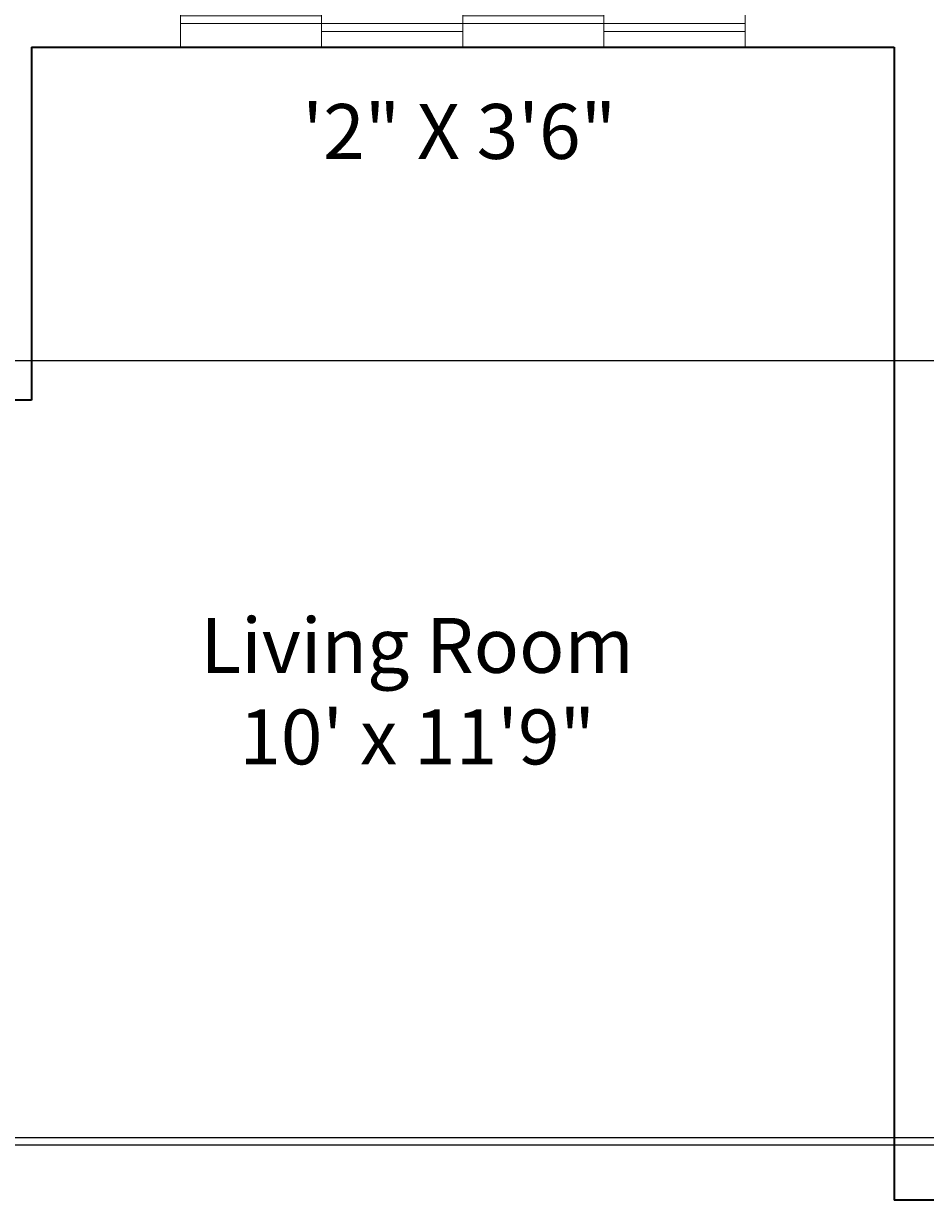
# Model space of a CAD drawing. Units: feet. Extents: x 105 to 1094, y -88 to 588.
# Tile 40 of 59: x 436 to 551, y 288 to 438. Entities that reach past the tile are written whole.
import ezdxf

# ---------------------------------------------------------------- set-up
doc = ezdxf.new("R2010")
doc.units = ezdxf.units.FT
doc.header["$MEASUREMENT"] = 0
for name, color, linetype, lineweight in [('A-ANNO-DIMS', 2, 'Continuous', 18), ('A-AREA-IDEN', 7, 'Continuous', 18), ('A-GLAZ', 4, 'Continuous', 18), ('A-WALL', 7, 'Continuous', 35)]:
    doc.layers.add(name, color=color, linetype=linetype, lineweight=lineweight)
doc.styles.get("Standard").update_dxf_attribs({"font": 'arial.ttf'})
doc.dimstyles.get("Standard").update_dxf_attribs({"dimtxt": 0.18, "dimasz": 0.18, "dimexe": 0.18, "dimexo": 0.0625, "dimgap": 0.09, "dimtad": 0, "dimtih": 1, "dimtoh": 1, "dimdec": 4, "dimzin": 0, "dimdsep": 46, "dimtxsty": 'Standard', "dimcen": 0.09, "dimadec": 0, "dimazin": 0, "dimtfac": 1, "dimtdec": 4, "dimtofl": 0, "dimtmove": 0, "dimatfit": 3, "dimfxl": 1, "dimtolj": 1, "dimtzin": 0, "dimarcsym": 0})

# ---------------------------------------------------------------- blocks, each defined once
blk = doc.blocks.new('WIN-FOUR-LIGHT-WIDE')
for p, q in [((0, 0), (0, 6)), ((18, 0), (18, 6)), ((36, 0), (36, 6)), ((54, 0), (54, 6)), ((72, 0), (72, 6)), ((18, 4), (36, 4)), ((54, 4), (72, 4)), ((0, 3), (72, 3)), ((0, 2), (18, 2)), ((36, 2), (54, 2))]:
    blk.add_line(p, q)
blk = doc.blocks.new('*D21')
at = {"layer": 'A-ANNO-DIMS', "color": 0, "lineweight": -2, "transparency": 16777216}
for p, q in [((849.63, 543.08), (105.46, 543.08)), ((105.64, 542.9), (105.64, 250.26)), ((105.64, -42.74), (105.64, 249.9)), ((849.63, -42.92), (105.46, -42.92))]:
    blk.add_line(p, q, dxfattribs=at)
at = {"layer": 'A-ANNO-DIMS', "color": 0, "transparency": 16777216}
for points in [[(105.61, 542.9), (105.67, 542.9), (105.64, 543.08)], [(105.61, -42.74), (105.67, -42.74), (105.64, -42.92)]]:
    blk.add_solid(points, dxfattribs=at)
at = {"layer": 'Defpoints', "color": 0, "transparency": 16777216}
for p in [(105.64, 543.08), (849.69, 543.08), (849.69, -42.92)]:
    blk.add_point(p, dxfattribs=at)
at = {"layer": 'A-ANNO-DIMS', "color": 0, "transparency": 16777216, "insert": (105.64, 250.08), "char_height": 0.18, "attachment_point": 5}
blk.add_mtext('\\A1;586', dxfattribs=at)
blk = doc.blocks.new('*D33')
at = {"layer": 'A-ANNO-DIMS', "color": 0, "lineweight": -2, "transparency": 16777216}
for p, q in [((646.63, 395.08), (105.46, 395.08)), ((105.64, 394.9), (105.64, 345.26)), ((105.64, 295.26), (105.64, 344.9)), ((646.63, 295.08), (105.46, 295.08))]:
    blk.add_line(p, q, dxfattribs=at)
at = {"layer": 'A-ANNO-DIMS', "color": 0, "transparency": 16777216}
for points in [[(105.61, 394.9), (105.67, 394.9), (105.64, 395.08)], [(105.61, 295.26), (105.67, 295.26), (105.64, 295.08)]]:
    blk.add_solid(points, dxfattribs=at)
at = {"layer": 'Defpoints', "color": 0, "transparency": 16777216}
for p in [(646.69, 395.08), (105.64, 295.08), (646.69, 295.08)]:
    blk.add_point(p, dxfattribs=at)
at = {"layer": 'A-ANNO-DIMS', "color": 0, "transparency": 16777216, "insert": (105.64, 345.08), "char_height": 0.18, "attachment_point": 5}
blk.add_mtext('\\A1;100', dxfattribs=at)
blk = doc.blocks.new('*D54')
at = {"layer": 'A-ANNO-DIMS', "color": 0, "lineweight": -2, "transparency": 16777216}
for p, q in [((294.75, 296.08), (1093.92, 296.08)), ((1093.74, 295.9), (1093.74, 286.26)), ((1093.74, 276.26), (1093.74, 285.9)), ((294.75, 276.08), (1093.92, 276.08))]:
    blk.add_line(p, q, dxfattribs=at)
at = {"layer": 'A-ANNO-DIMS', "color": 0, "transparency": 16777216}
for points in [[(1093.71, 295.9), (1093.77, 295.9), (1093.74, 296.08)], [(1093.71, 276.26), (1093.77, 276.26), (1093.74, 276.08)]]:
    blk.add_solid(points, dxfattribs=at)
at = {"layer": 'Defpoints', "color": 0, "transparency": 16777216}
for p in [(294.69, 296.08), (1093.74, 296.08), (294.69, 276.08)]:
    blk.add_point(p, dxfattribs=at)
at = {"layer": 'A-ANNO-DIMS', "color": 0, "transparency": 16777216, "insert": (1093.74, 286.08), "char_height": 0.18, "attachment_point": 5}
blk.add_mtext('\\A1;20', dxfattribs=at)

msp = doc.modelspace()

# ---------------------------------------------------------------- linework, layer by layer
at = {"layer": 'A-WALL'}
for p, q in [((436.6883, 435.0812), (546.6883, 435.0812)), ((436.6883, 435.0812), (436.6883, 390.0812)), ((546.6883, 435.0812), (546.6883, 288.0812)), ((436.6883, 390.0812), (414.6883, 390.0812)), ((552.6883, 288.0812), (546.6883, 288.0812))]:
    msp.add_line(p, q, dxfattribs=at)

# ---------------------------------------------------------------- block references
at = {"layer": 'A-GLAZ', "extrusion": (0, 0, -1), "zscale": -1, "rotation": 180}
msp.add_blockref('WIN-FOUR-LIGHT-WIDE', (-455.688, 441.0813), dxfattribs=at)

# ---------------------------------------------------------------- texts
at = {"layer": 'A-ANNO-DIMS', "insert": (540.4102, 427.8248), "char_height": 7, "attachment_point": 3}
msp.add_mtext_dynamic_manual_height_columns('\\pxqc;\'2" X 3\'6"', width=98.34246, gutter_width=1, heights=[0], dxfattribs=at)
at = {"layer": 'A-AREA-IDEN', "insert": (535.0519, 362.3098), "char_height": 7, "attachment_point": 3}
msp.add_mtext_dynamic_manual_height_columns('\\pxqc;Living Room \\P10\' x 11\'9"', width=98.34246, gutter_width=1, heights=[0], dxfattribs=at)

# ---------------------------------------------------------------- dimensions: what is measured, and where the dimension line sits
at = {"layer": 'A-ANNO-DIMS'}
for base, p1, p2, picture, middle in [((105.6383, 543.0812), (849.6883, -42.9188), (849.6883, 543.0812), '*D21', (105.6383, 250.0812)), ((105.6383, 295.0812), (646.6883, 395.0812), (646.6883, 295.0812), '*D33', (105.6383, 345.0812)), ((1093.7383, 296.0812), (294.6883, 276.0812), (294.6883, 296.0812), '*D54', (1093.7383, 286.0812))]:
    dim = msp.add_linear_dim(base=base, p1=p1, p2=p2, angle=90, dimstyle='Standard', override={"dimdec": 0, "dimlfac": 1, "dimrnd": 0, "dimzin": 0, "dimdsep": 46, "dimlunit": 2}, dxfattribs=at)
    dim.commit()
    dim.dimension.update_dxf_attribs({"geometry": picture, "text_midpoint": middle})

doc.saveas('drawing.dxf')
